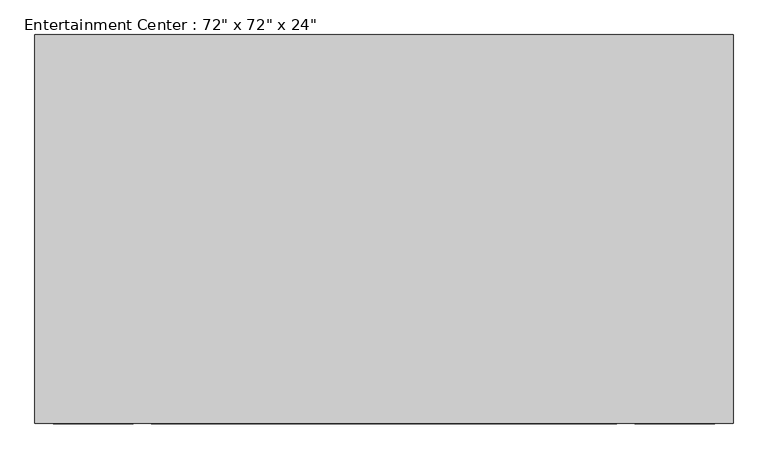
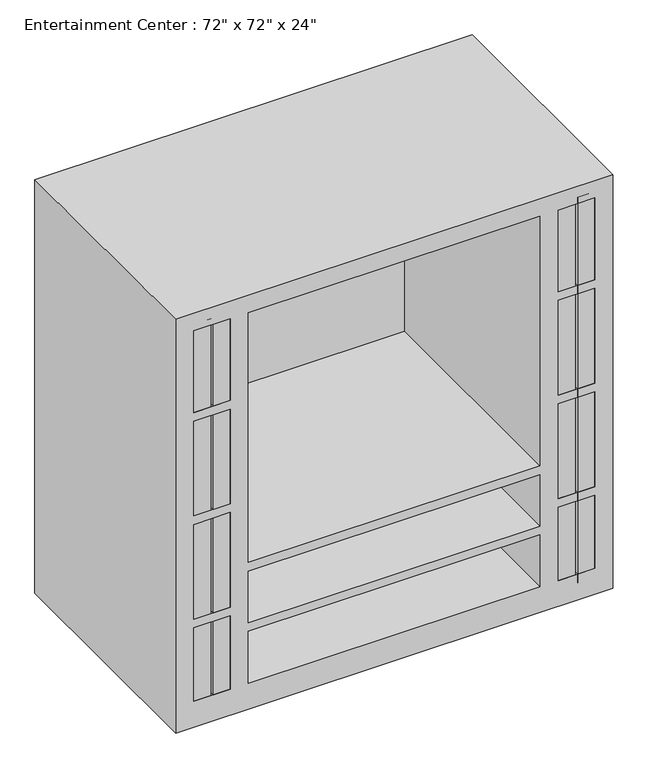
"""IFC4 building model written with IfcOpenShell, lengths in millimetres: furniture geometry."""

from ifc_helpers import new_model, si_unit, point, frame, frame_2d, origin, place, context, project, spatial, polyline, circle_curve, trimmed, segment, composite_curve, outline, extrude, faceted_brep, source, transform, mapped, element, save


def furniture_80f2079a(model_context):
    return source(origin(), model_context, "Body", "SolidModel", [
        faceted_brep([(609.6, -781.05, 0.0), (609.6, -781.05, 1219.2), (-609.6, -781.05, 1219.2), (-609.6, -781.05, 0.0), (-457.2, -781.05, 1168.4), (-457.2, -781.05, 927.1), (-558.8, -781.05, 927.1), (-558.8, -781.05, 1168.4), (-457.2, -781.05, 76.2), (-558.8, -781.05, 76.2), (-558.8, -781.05, 292.1), (-457.2, -781.05, 292.1), (558.8, -781.05, 927.1), (457.2, -781.05, 927.1), (457.2, -781.05, 1168.4), (558.8, -781.05, 1168.4), (-406.4, -781.05, 431.8), (-406.4, -781.05, 1168.4), (406.4, -781.05, 1168.4), (406.4, -781.05, 431.8), (406.4, -781.05, 76.2), (-406.4, -781.05, 76.2), (-406.4, -781.05, 228.6), (406.4, -781.05, 228.6), (558.8, -781.05, 76.2), (457.2, -781.05, 76.2), (457.2, -781.05, 292.1), (558.8, -781.05, 292.1), (-558.8, -781.05, 317.5), (-558.8, -781.05, 596.9), (-457.2, -781.05, 596.9), (-457.2, -781.05, 317.5), (-457.2, -781.05, 901.7), (-457.2, -781.05, 622.3), (-558.8, -781.05, 622.3), (-558.8, -781.05, 901.7), (457.2, -781.05, 901.7), (558.8, -781.05, 901.7), (558.8, -781.05, 622.3), (457.2, -781.05, 622.3), (457.2, -781.05, 596.9), (558.8, -781.05, 596.9), (558.8, -781.05, 317.5), (457.2, -781.05, 317.5), (406.4, -781.05, 254.0), (-406.4, -781.05, 254.0), (-406.4, -781.05, 406.4), (406.4, -781.05, 406.4), (609.6, -101.6, 0.0), (-609.6, -101.6, 0.0), (-609.6, -101.6, 1219.2), (609.6, -101.6, 1219.2), (-457.2, -127.0, 1168.4), (-457.2, -127.0, 927.1), (-558.8, -127.0, 927.1), (-558.8, -127.0, 1168.4), (-457.2, -127.0, 76.2), (-558.8, -127.0, 76.2), (-558.8, -127.0, 292.1), (-457.2, -127.0, 292.1), (558.8, -127.0, 927.1), (457.2, -127.0, 927.1), (457.2, -127.0, 1168.4), (558.8, -127.0, 1168.4), (-406.4, -127.0, 431.8), (-406.4, -127.0, 1168.4), (406.4, -127.0, 1168.4), (406.4, -127.0, 431.8), (406.4, -127.0, 76.2), (-406.4, -127.0, 76.2), (-406.4, -127.0, 228.6), (406.4, -127.0, 228.6), (558.8, -127.0, 76.2), (457.2, -127.0, 76.2), (457.2, -127.0, 292.1), (558.8, -127.0, 292.1), (-558.8, -127.0, 317.5), (-558.8, -127.0, 596.9), (-457.2, -127.0, 596.9), (-457.2, -127.0, 317.5), (-457.2, -127.0, 901.7), (-457.2, -127.0, 622.3), (-558.8, -127.0, 622.3), (-558.8, -127.0, 901.7), (457.2, -127.0, 901.7), (558.8, -127.0, 901.7), (558.8, -127.0, 622.3), (457.2, -127.0, 622.3), (457.2, -127.0, 596.9), (558.8, -127.0, 596.9), (558.8, -127.0, 317.5), (457.2, -127.0, 317.5), (406.4, -127.0, 254.0), (-406.4, -127.0, 254.0), (-406.4, -127.0, 406.4), (406.4, -127.0, 406.4)], [[[0, 1, 2, 3], [4, 5, 6, 7], [8, 9, 10, 11], [12, 13, 14, 15], [16, 17, 18, 19], [20, 21, 22, 23], [24, 25, 26, 27], [28, 29, 30, 31], [32, 33, 34, 35], [36, 37, 38, 39], [40, 41, 42, 43], [44, 45, 46, 47]], [[48, 49, 50, 51]], [[1, 0, 48, 51]], [[2, 1, 51, 50]], [[3, 2, 50, 49]], [[0, 3, 49, 48]], [[5, 4, 52, 53]], [[6, 5, 53, 54]], [[7, 6, 54, 55]], [[4, 7, 55, 52]], [[9, 8, 56, 57]], [[10, 9, 57, 58]], [[11, 10, 58, 59]], [[8, 11, 59, 56]], [[13, 12, 60, 61]], [[14, 13, 61, 62]], [[15, 14, 62, 63]], [[12, 15, 63, 60]], [[17, 16, 64, 65]], [[18, 17, 65, 66]], [[19, 18, 66, 67]], [[16, 19, 67, 64]], [[21, 20, 68, 69]], [[22, 21, 69, 70]], [[23, 22, 70, 71]], [[20, 23, 71, 68]], [[25, 24, 72, 73]], [[26, 25, 73, 74]], [[27, 26, 74, 75]], [[24, 27, 75, 72]], [[29, 28, 76, 77]], [[30, 29, 77, 78]], [[31, 30, 78, 79]], [[28, 31, 79, 76]], [[33, 32, 80, 81]], [[34, 33, 81, 82]], [[35, 34, 82, 83]], [[32, 35, 83, 80]], [[37, 36, 84, 85]], [[38, 37, 85, 86]], [[39, 38, 86, 87]], [[36, 39, 87, 84]], [[41, 40, 88, 89]], [[42, 41, 89, 90]], [[43, 42, 90, 91]], [[40, 43, 91, 88]], [[45, 44, 92, 93]], [[46, 45, 93, 94]], [[47, 46, 94, 95]], [[44, 47, 95, 92]], [[53, 52, 55, 54]], [[57, 56, 59, 58]], [[61, 60, 63, 62]], [[65, 64, 67, 66]], [[69, 68, 71, 70]], [[73, 72, 75, 74]], [[77, 76, 79, 78]], [[81, 80, 83, 82]], [[85, 84, 87, 86]], [[89, 88, 91, 90]], [[93, 92, 95, 94]]]),
        extrude(outline(composite_curve([segment(polyline([(698.5, -480.5986452), (698.5, -504.825), (520.7, -504.825), (520.7, -480.5986452)]), True, "CONTINUOUS"), segment(trimmed(circle_curve(frame_2d((546.1, -480.5986452)), 25.4), [point((520.7, -480.5986452))], [point((546.1, -455.1986452))], False, "CARTESIAN"), True, "CONTINUOUS"), segment(polyline([(546.1, -455.1986452), (673.1, -455.1986452)]), True, "CONTINUOUS"), segment(trimmed(circle_curve(frame_2d((673.1, -480.5986452)), 25.4), [point((673.1, -455.1986452))], [point((698.5, -480.5986452))], False, "CARTESIAN"), True, "CONTINUOUS")], self_intersect=False)), frame((0.0, -714.375, 0.0), z_axis=(0.0, 1.0, 0.0), x_axis=(0.0, 0.0, 1.0)), (0.0, 0.0, 1.0), 3.175),
        extrude(outline(composite_curve([segment(trimmed(circle_curve(frame_2d((673.1, -535.78125)), 25.4), [point((698.5, -535.78125))], [point((673.1, -561.18125))], False, "CARTESIAN"), True, "CONTINUOUS"), segment(polyline([(673.1, -561.18125), (546.1, -561.18125)]), True, "CONTINUOUS"), segment(trimmed(circle_curve(frame_2d((546.1, -535.78125)), 25.4), [point((546.1, -561.18125))], [point((520.7, -535.78125))], False, "CARTESIAN"), True, "CONTINUOUS"), segment(polyline([(520.7, -535.78125), (520.7, -511.175), (698.5, -511.175), (698.5, -535.78125)]), True, "CONTINUOUS")], self_intersect=False)), frame((0.0, -714.375, 0.0), z_axis=(0.0, 1.0, 0.0), x_axis=(0.0, 0.0, 1.0)), (0.0, 0.0, 1.0), 3.175),
        extrude(outline(composite_curve([segment(trimmed(circle_curve(frame_2d((673.1, 480.5986452)), 25.4), [point((698.5, 480.5986452))], [point((673.1, 455.1986452))], False, "CARTESIAN"), True, "CONTINUOUS"), segment(polyline([(673.1, 455.1986452), (546.1, 455.1986452)]), True, "CONTINUOUS"), segment(trimmed(circle_curve(frame_2d((546.1, 480.5986452)), 25.4), [point((546.1, 455.1986452))], [point((520.7, 480.5986452))], False, "CARTESIAN"), True, "CONTINUOUS"), segment(polyline([(520.7, 480.5986452), (520.7, 504.825), (698.5, 504.825), (698.5, 480.5986452)]), True, "CONTINUOUS")], self_intersect=False)), frame((0.0, -714.375, 0.0), z_axis=(0.0, 1.0, 0.0), x_axis=(0.0, 0.0, 1.0)), (0.0, 0.0, 1.0), 3.175),
        extrude(outline(composite_curve([segment(polyline([(698.5, 535.78125), (698.5, 511.175), (520.7, 511.175), (520.7, 535.78125)]), True, "CONTINUOUS"), segment(trimmed(circle_curve(frame_2d((546.1, 535.78125)), 25.4), [point((520.7, 535.78125))], [point((546.1, 561.18125))], False, "CARTESIAN"), True, "CONTINUOUS"), segment(polyline([(546.1, 561.18125), (673.1, 561.18125)]), True, "CONTINUOUS"), segment(trimmed(circle_curve(frame_2d((673.1, 535.78125)), 25.4), [point((673.1, 561.18125))], [point((698.5, 535.78125))], False, "CARTESIAN"), True, "CONTINUOUS")], self_intersect=False)), frame((0.0, -714.375, 0.0), z_axis=(0.0, 1.0, 0.0), x_axis=(0.0, 0.0, 1.0)), (0.0, 0.0, 1.0), 3.175),
        extrude(outline(polyline([(-577.85, -711.2), (-511.175, -711.2), (-511.175, -781.05), (-577.85, -781.05), (-577.85, -711.2)])), frame((0.0, 0.0, 50.8), z_axis=(0.0, 0.0, 1.0), x_axis=(1.0, 0.0, 0.0)), (0.0, 0.0, 1.0), 1136.65),
        extrude(outline(polyline([(-504.825, -711.2), (-438.15, -711.2), (-438.15, -781.05), (-504.825, -781.05), (-504.825, -711.2)])), frame((0.0, 0.0, 50.8), z_axis=(0.0, 0.0, 1.0), x_axis=(1.0, 0.0, 0.0)), (0.0, 0.0, 1.0), 1136.65),
        extrude(outline(polyline([(511.175, -711.2), (577.85, -711.2), (577.85, -781.05), (511.175, -781.05), (511.175, -711.2)])), frame((0.0, 0.0, 50.8), z_axis=(0.0, 0.0, 1.0), x_axis=(1.0, 0.0, 0.0)), (0.0, 0.0, 1.0), 1136.65),
        extrude(outline(polyline([(438.15, -711.2), (504.825, -711.2), (504.825, -781.05), (438.15, -781.05), (438.15, -711.2)])), frame((0.0, 0.0, 50.8), z_axis=(0.0, 0.0, 1.0), x_axis=(1.0, 0.0, 0.0)), (0.0, 0.0, 1.0), 1136.65),
    ])


if __name__ == "__main__":
    model = new_model("IFC4")
    model_context = context("Model", 3, world=origin())
    ifc_project = project(units=[si_unit("LENGTHUNIT", "METRE", prefix="MILLI")], contexts=[model_context])
    site = spatial("IfcSite", under=ifc_project)
    building = spatial("IfcBuilding", under=site)
    placement = place(None, origin())
    furniture_shape = furniture_80f2079a(model_context)
    element("IfcFurniture", 1, ObjectType="Entertainment Center : 72\" x 72\" x 24\"", at=placement, inside=building, context=model_context, shape_type="MappedRepresentation", body=[
        mapped(furniture_shape, transform((0.0, 0.0, 0.0), x_axis=(1.0, 0.0, 0.0), y_axis=(0.0, 1.0, 0.0), z_axis=(0.0, 0.0, 1.0))),
    ])
    save(model, "model.ifc")

# Revit data of these elements
# Type "Entertainment Center : 72\" x 72\" x 24\""
#   Assembly Code = "E2020200"
#   Center Width = 2' - 8"
#   Depth = 2' - 0"
#   Height = 4' - 0"
#   Width = 4' - 0"
#   Material = none
#   Default Elevation = 0
# Element 1 (IfcFurniture, "Entertainment Center : 72\" x 72\" x 24\"")
#   Materials on its faces: "Steel, Chrome Plated", "Glass - Clear, Grey"
# Materials
#   "Steel, Chrome Plated": class "Metal", colour RGB 17 17 17, transparency 0, Description = "Chromiuim plated steel", Cost = 0
#   "Glass - Clear, Grey": class "Glass", colour RGB 252 255 255, transparency 0.64
